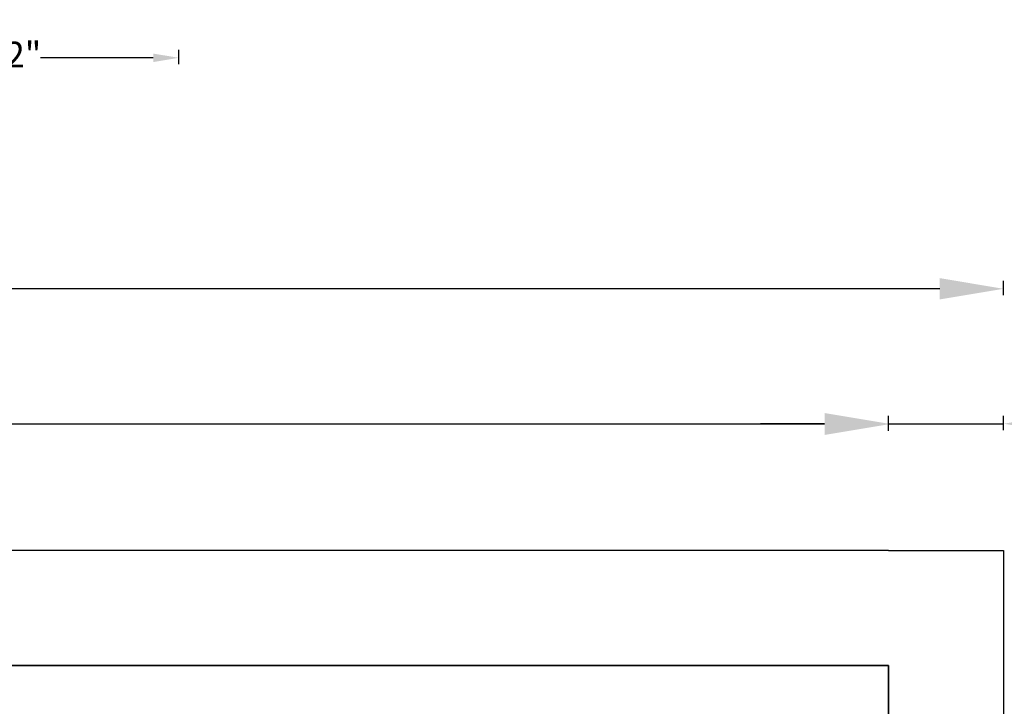
# Model space of a CAD drawing. Units: inches. Extents: x -638 to 186, y -762 to 59.
# Tile 30 of 31: x -125 to 29, y -48 to 59. Entities that reach past the tile are written whole.
import ezdxf

# ---------------------------------------------------------------- set-up
doc = ezdxf.new("R2010")
doc.units = ezdxf.units.IN
for name, color, linetype, lineweight in [('A-ANNO-DIMS', 2, 'Continuous', 18), ('C-PROP', 7, 'Continuous', 25), ('wall', 7, 'Continuous', 35)]:
    doc.layers.add(name, color=color, linetype=linetype, lineweight=lineweight)
doc.styles.get("Standard").update_dxf_attribs({"font": 'arial.ttf'})
doc.dimstyles.new('ISO-25', dxfattribs={"dimtxt": 4, "dimasz": 4, "dimexe": 1.25, "dimexo": 0.625, "dimtad": 0, "dimlunit": 4, "dimtxsty": 'Standard', "dimcen": 2.5, "dimclrt": 256, "dimadec": 0, "dimazin": 0, "dimtfac": 1, "dimtmove": 0, "dimatfit": 3, "dimfxl": 1, "dimfxlon": 1, "dimarcsym": 0})

# ---------------------------------------------------------------- blocks, each defined once
blk = doc.blocks.new('*D9')
at = {"layer": 'A-ANNO-DIMS', "color": 0, "lineweight": -2, "transparency": 16777216}
for p, q in [((-413.53, -5.3), (-413.53, -3.05)), ((10.47, -5.3), (10.47, -3.05)), ((-403.53, -4.3), (-219.32, -4.3)), ((0.47, -4.3), (-183.73, -4.3))]:
    blk.add_line(p, q, dxfattribs=at)
at = {"layer": 'A-ANNO-DIMS', "color": 0, "lineweight": 30, "transparency": 16777216}
for points in [[(-403.53, -2.64), (-403.53, -5.97), (-413.53, -4.3)], [(0.47, -2.64), (0.47, -5.97), (10.47, -4.3)]]:
    blk.add_solid(points, dxfattribs=at)
at = {"layer": 'Defpoints', "color": 0, "lineweight": 30, "transparency": 16777216}
for p in [(10.47, -4.3), (-413.53, -42.03), (10.47, -42.03)]:
    blk.add_point(p, dxfattribs=at)
at = {"layer": 'A-ANNO-DIMS', "color": 0, "transparency": 16777216, "insert": (-201.53, -4.3), "char_height": 10, "attachment_point": 5}
blk.add_mtext('35\'-4"', dxfattribs=at)
blk = doc.blocks.new('*D10')
at = {"layer": 'A-ANNO-DIMS', "color": 0, "lineweight": -2, "transparency": 16777216}
for p, q in [((10.47, -5.21), (10.47, -2.96)), ((28.47, -5.21), (28.47, -2.96)), ((0.47, -4.21), (-9.53, -4.21)), ((10.47, -4.21), (28.47, -4.21)), ((38.47, -4.21), (48.47, -4.21))]:
    blk.add_line(p, q, dxfattribs=at)
at = {"layer": 'A-ANNO-DIMS', "color": 0, "lineweight": 30, "transparency": 16777216}
for points in [[(0.47, -2.54), (0.47, -5.88), (10.47, -4.21)], [(38.47, -2.54), (38.47, -5.88), (28.47, -4.21)]]:
    blk.add_solid(points, dxfattribs=at)
at = {"layer": 'Defpoints', "color": 0, "lineweight": 30, "transparency": 16777216}
for p in [(28.47, -4.21), (10.47, -42.03), (28.47, -42.03)]:
    blk.add_point(p, dxfattribs=at)
at = {"layer": 'A-ANNO-DIMS', "color": 0, "transparency": 16777216, "insert": (61.92, -4.21), "char_height": 10, "attachment_point": 5}
blk.add_mtext('1\'-6"', dxfattribs=at)
blk = doc.blocks.new('*D11')
at = {"layer": 'A-ANNO-DIMS', "color": 0, "lineweight": -2, "transparency": 16777216}
for p, q in [((-455.53, 15.89), (-455.53, 18.14)), ((28.47, 15.89), (28.47, 18.14)), ((-445.53, 16.89), (-231.53, 16.89)), ((18.47, 16.89), (-195.52, 16.89))]:
    blk.add_line(p, q, dxfattribs=at)
at = {"layer": 'A-ANNO-DIMS', "color": 0, "lineweight": 30, "transparency": 16777216}
for points in [[(-445.53, 18.56), (-445.53, 15.23), (-455.53, 16.89)], [(18.47, 18.56), (18.47, 15.23), (28.47, 16.89)]]:
    blk.add_solid(points, dxfattribs=at)
at = {"layer": 'Defpoints', "color": 0, "lineweight": 30, "transparency": 16777216}
for p in [(28.47, 16.89), (-455.53, -42.03), (28.47, -42.03)]:
    blk.add_point(p, dxfattribs=at)
at = {"layer": 'A-ANNO-DIMS', "color": 0, "transparency": 16777216, "insert": (-213.53, 16.89), "char_height": 10, "attachment_point": 5}
blk.add_mtext('40\'-4"', dxfattribs=at)
blk = doc.blocks.new('*D13')
at = {"layer": 'A-ANNO-DIMS', "color": 0, "lineweight": -2, "transparency": 16777216}
for p, q in [((46.29, -14.03), (46.29, -4.03)), ((45.29, -24.03), (47.54, -24.03)), ((46.29, -42.03), (46.29, -24.03)), ((46.29, -42.03), (46.29, -24.03)), ((63.79, -27.78), (63.79, -26.53)), ((46.29, -33.03), (63.79, -27.78)), ((45.29, -42.03), (47.54, -42.03)), ((46.29, -52.03), (46.29, -62.03))]:
    blk.add_line(p, q, dxfattribs=at)
at = {"layer": 'A-ANNO-DIMS', "color": 0, "lineweight": 30, "transparency": 16777216}
for points in [[(44.62, -14.03), (47.95, -14.03), (46.29, -24.03)], [(44.62, -52.03), (47.95, -52.03), (46.29, -42.03)]]:
    blk.add_solid(points, dxfattribs=at)
at = {"layer": 'Defpoints', "color": 0, "lineweight": 30, "transparency": 16777216}
for p in [(10.47, -24.03), (46.29, -24.03), (10.47, -42.03)]:
    blk.add_point(p, dxfattribs=at)
at = {"layer": 'A-ANNO-DIMS', "color": 0, "transparency": 16777216, "insert": (63.79, -13.09), "char_height": 10, "attachment_point": 5, "rotation": 90}
blk.add_mtext('1\'-6"', dxfattribs=at)
blk = doc.blocks.new('*D14')
at = {"layer": 'A-ANNO-DIMS', "color": 0, "lineweight": -2, "transparency": 16777216}
for p, q in [((45.41, -42.03), (47.66, -42.03)), ((46.41, -52.03), (46.41, -307.65)), ((46.41, -607.03), (46.41, -351.42)), ((45.41, -617.03), (47.66, -617.03))]:
    blk.add_line(p, q, dxfattribs=at)
at = {"layer": 'A-ANNO-DIMS', "color": 0, "lineweight": 30, "transparency": 16777216}
for points in [[(44.74, -52.03), (48.08, -52.03), (46.41, -42.03)], [(44.74, -607.03), (48.08, -607.03), (46.41, -617.03)]]:
    blk.add_solid(points, dxfattribs=at)
at = {"layer": 'Defpoints', "color": 0, "lineweight": 30, "transparency": 16777216}
for p in [(10.47, -42.03), (10.47, -617.03), (46.41, -617.03)]:
    blk.add_point(p, dxfattribs=at)
at = {"layer": 'A-ANNO-DIMS', "color": 0, "transparency": 16777216, "insert": (46.41, -329.53), "char_height": 10, "attachment_point": 5, "rotation": 90}
blk.add_mtext('47\'-11"', dxfattribs=at)
blk = doc.blocks.new('*D15')
at = {"layer": 'A-ANNO-DIMS', "color": 0, "lineweight": -2, "transparency": 16777216}
for p, q in [((69.33, -24.03), (71.58, -24.03)), ((70.33, -34.03), (70.33, -350.73)), ((70.33, -703.03), (70.33, -386.33)), ((69.33, -713.03), (71.58, -713.03))]:
    blk.add_line(p, q, dxfattribs=at)
at = {"layer": 'A-ANNO-DIMS', "color": 0, "lineweight": 30, "transparency": 16777216}
for points in [[(68.66, -34.03), (72, -34.03), (70.33, -24.03)], [(68.66, -703.03), (72, -703.03), (70.33, -713.03)]]:
    blk.add_solid(points, dxfattribs=at)
at = {"layer": 'Defpoints', "color": 0, "lineweight": 30, "transparency": 16777216}
for p in [(-24.67, -24.03), (-10.56, -713.03), (70.33, -713.03)]:
    blk.add_point(p, dxfattribs=at)
at = {"layer": 'A-ANNO-DIMS', "color": 0, "transparency": 16777216, "insert": (70.33, -368.53), "char_height": 10, "attachment_point": 5, "rotation": 90}
blk.add_mtext('57\'-5"', dxfattribs=at)
blk = doc.blocks.new('*D56')
at = {"layer": 'A-ANNO-DIMS', "color": 0, "lineweight": -2, "transparency": 16777216}
for p, q in [((-165.03, 52.02), (-165.03, 54.27)), ((-100.53, 52.02), (-100.53, 54.27)), ((-161.03, 53.02), (-143.38, 53.02)), ((-104.53, 53.02), (-122.17, 53.02))]:
    blk.add_line(p, q, dxfattribs=at)
at = {"layer": 'A-ANNO-DIMS', "color": 0, "lineweight": 30, "transparency": 16777216}
for points in [[(-161.03, 53.68), (-161.03, 52.35), (-165.03, 53.02)], [(-104.53, 53.68), (-104.53, 52.35), (-100.53, 53.02)]]:
    blk.add_solid(points, dxfattribs=at)
at = {"layer": 'Defpoints', "color": 0, "lineweight": 30, "transparency": 16777216}
for p in [(-100.53, 53.02), (-165.03, -408.03), (-100.53, -408.03)]:
    blk.add_point(p, dxfattribs=at)
at = {"layer": 'A-ANNO-DIMS', "transparency": 16777216, "insert": (-132.78, 53.02), "char_height": 4, "attachment_point": 5}
blk.add_mtext('5\'-4 1/2"', dxfattribs=at)

msp = doc.modelspace()

# ---------------------------------------------------------------- linework, layer by layer
at = {"layer": 'C-PROP'}
for p, q in [((10.474, -24.033), (-468.465, -24.033)), ((10.474, -24.033), (28.474, -24.033)), ((28.474, -24.033), (28.474, -713.033))]:
    msp.add_line(p, q, dxfattribs=at)
at = {"layer": 'wall'}
for p, q in [((-223.526, -42.033), (10.474, -42.033)), ((10.474, -42.033), (10.474, -617.033))]:
    msp.add_line(p, q, dxfattribs=at)

# ---------------------------------------------------------------- dimensions: what is measured, and where the dimension line sits
at = {"layer": 'A-ANNO-DIMS'}
for base, p1, p2, override, picture, middle in [((-100.526, 53.017), (-165.026, -408.033), (-100.526, -408.033), {"dimdec": 1, "dimlfac": 1, "dimrnd": 0, "dimzin": 1, "dimdsep": 46, "dimlunit": 4, "dimfrac": 2}, '*D56', (-132.776, 53.017)), ((28.474, 16.893), (-455.526, -42.033), (28.474, -42.033), {"dimtxt": 10, "dimasz": 10, "dimclrd": 0, "dimclre": 0, "dimclrt": 0}, '*D11', (-213.526, 16.893)), ((10.474, -4.303), (-413.526, -42.033), (10.474, -42.033), {"dimtxt": 10, "dimasz": 10, "dimclrd": 0, "dimclre": 0, "dimclrt": 0}, '*D9', (-201.526, -4.303)), ((28.474, -4.209), (10.474, -42.033), (28.474, -42.033), {"dimtxt": 10, "dimasz": 10, "dimclrd": 0, "dimclre": 0, "dimclrt": 0}, '*D10', (61.92, -4.209))]:
    dim = msp.add_linear_dim(base=base, p1=p1, p2=p2, dimstyle='ISO-25', override=override, dxfattribs=at)
    dim.commit()
    dim.dimension.update_dxf_attribs({"geometry": picture, "text_midpoint": middle})
for base, p1, p2, override, picture, middle in [((46.286, -24.033), (10.474, -42.033), (10.474, -24.033), {"dimtxt": 10, "dimasz": 10, "dimclrd": 0, "dimclre": 0, "dimclrt": 0, "dimtmove": 1}, '*D13', (63.791, -25.907)), ((70.331, -713.033), (-24.669, -24.033), (-10.563, -713.033), {"dimtxt": 10, "dimasz": 10, "dimclrd": 0, "dimclre": 0, "dimclrt": 0}, '*D15', (70.331, -368.533)), ((46.411, -617.033), (10.474, -42.033), (10.474, -617.033), {"dimtxt": 10, "dimasz": 10, "dimclrd": 0, "dimclre": 0, "dimclrt": 0}, '*D14', (46.411, -329.533))]:
    dim = msp.add_linear_dim(base=base, p1=p1, p2=p2, angle=90, dimstyle='ISO-25', override=override, dxfattribs=at)
    dim.commit()
    dim.dimension.update_dxf_attribs({"geometry": picture, "text_midpoint": middle})

doc.saveas('drawing.dxf')
